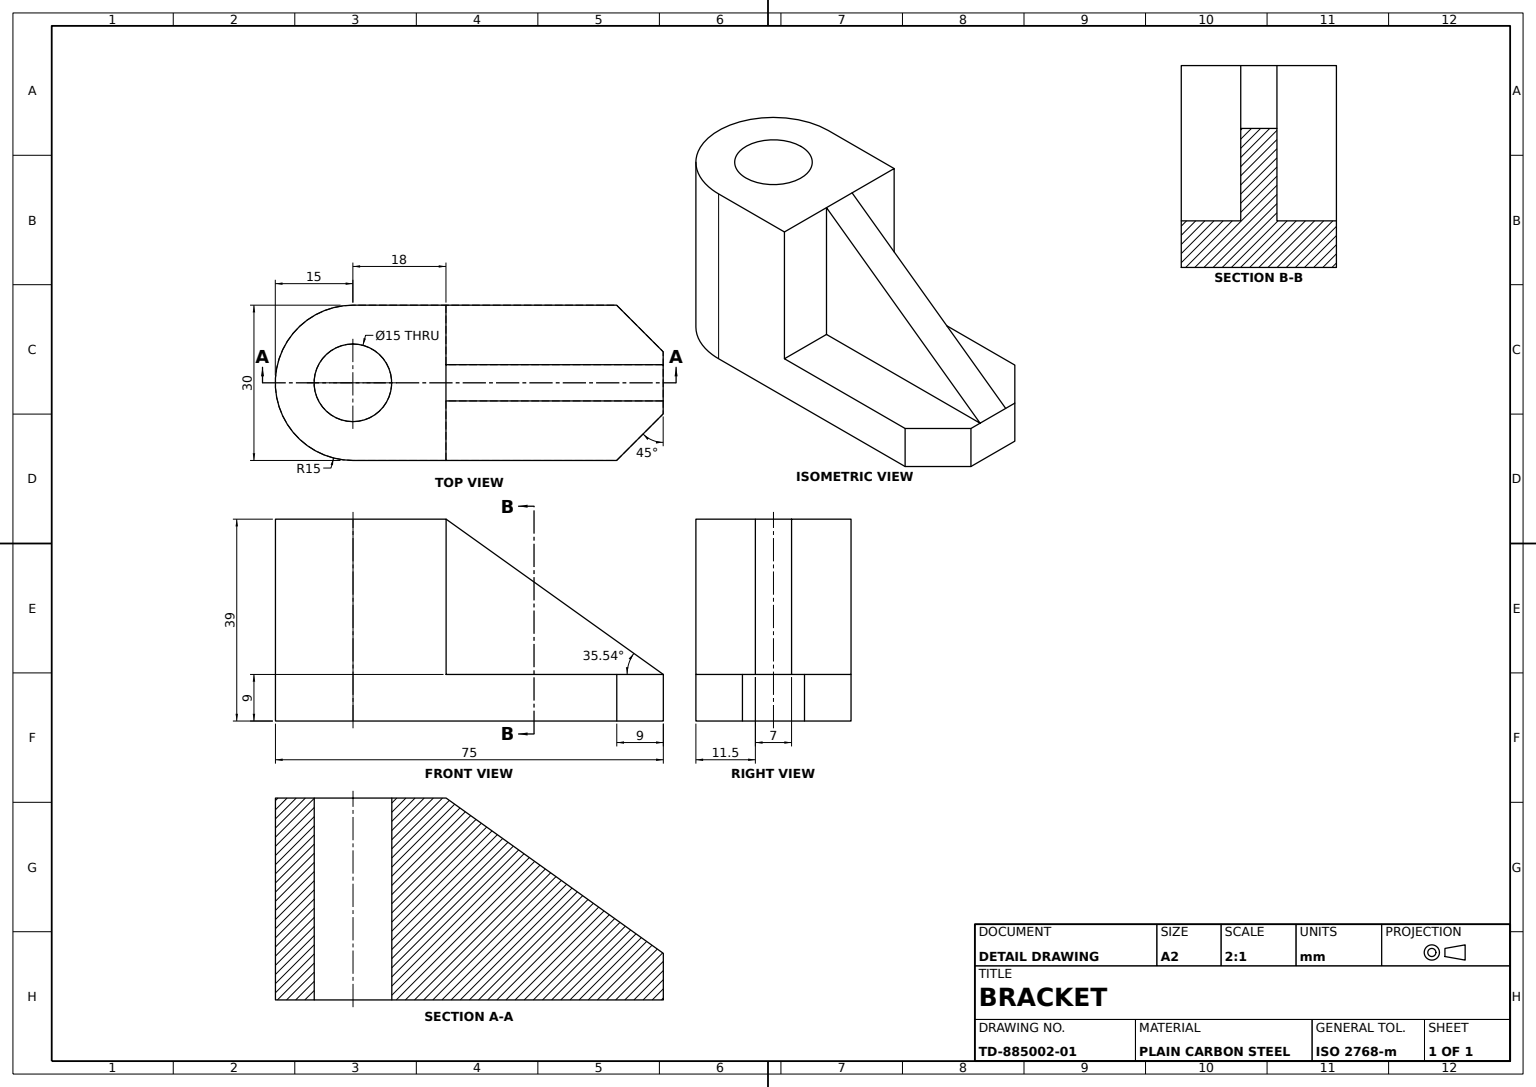
from build123d import *

# Parameters (mm, degrees)
BASE_PLATE_DEPTH      = 9
BASE_END_CUT_DEPTH    = 9
UPRIGHT_START         = 30
UPRIGHT_BOSS_SKETCH_R = 7.5
UPRIGHT_BOSS_DEPTH    = 30
SUPPORT_RIB_DEPTH     = 3.5
BOSS_BORE_SKETCH_R    = 7.5
BOSS_BORE_DEPTH       = 57.144901817


with BuildPart() as part:
    # Base Plate Sketch → Base Plate (new body)
    with BuildSketch(Plane(origin=(0, 0, 0), x_dir=(1, 0, 0), z_dir=(0, 1, 0))):
        Polygon((28.5, 15), (37.5, 6), (37.5, -6), (28.5, -15), (-37.5, -15), (-37.5, 15), align=None)
    extrude(amount=BASE_PLATE_DEPTH)

    # Base End Cut Sketch → Base End Cut (cut)
    with BuildSketch(Plane(origin=(0, 9, 0), x_dir=(1, 0, 0), z_dir=(0, 1, 0))):
        with BuildLine():
            Line((-37.5, 1.12e-07), (-37.5, -15))
            Line((-37.5, -15), (-22.5, -15))
            ThreePointArc((-22.5, -15), (-33.106601757, -10.606601678), (-37.5, 1.12e-07))
        make_face()
        with BuildLine():
            Line((-37.5, 15), (-37.5, 1.12e-07))
            ThreePointArc((-37.5, 1.12e-07), (-33.106601678, 10.606601757), (-22.5, 15))
            Line((-22.5, 15), (-37.5, 15))
        make_face()
    extrude(amount=-BASE_END_CUT_DEPTH, mode=Mode.SUBTRACT)

    # Upright Boss Sketch → Upright Boss (add)
    with BuildSketch(Plane(origin=(0, 9, 0), x_dir=(1, 0, 0), z_dir=(0, 1, 0)).offset(UPRIGHT_START)):
        with BuildLine():
            Line((-4.5, 15), (-22.5, 15))
            ThreePointArc((-22.5, 15), (-37.5, 0), (-22.5, -15))
            Line((-22.5, -15), (-4.5, -15))
            Line((-4.5, -15), (-4.5, 15))
        make_face()
        with Locations(Location((-22.5, 0, 0), (0, 0, 270))):
            Circle(UPRIGHT_BOSS_SKETCH_R, mode=Mode.SUBTRACT)
    extrude(amount=-UPRIGHT_BOSS_DEPTH)

    # Support Rib Sketch → Support Rib (add, symmetric)
    with BuildSketch(Plane.XY):
        Polygon((-4.5, 39), (37.5, 9), (-4.5, 9), align=None)
    extrude(amount=SUPPORT_RIB_DEPTH, both=True)

    # Boss Bore Sketch → Boss Bore (cut, through all)
    with BuildSketch(Plane(origin=(0, 39, 0), x_dir=(1, 0, 0), z_dir=(0, 1, 0))):
        with Locations(Location((-22.5, 0, 0), (0, 0, 270))):
            Circle(BOSS_BORE_SKETCH_R)
    extrude(amount=-BOSS_BORE_DEPTH, mode=Mode.SUBTRACT)


solid = part.part
